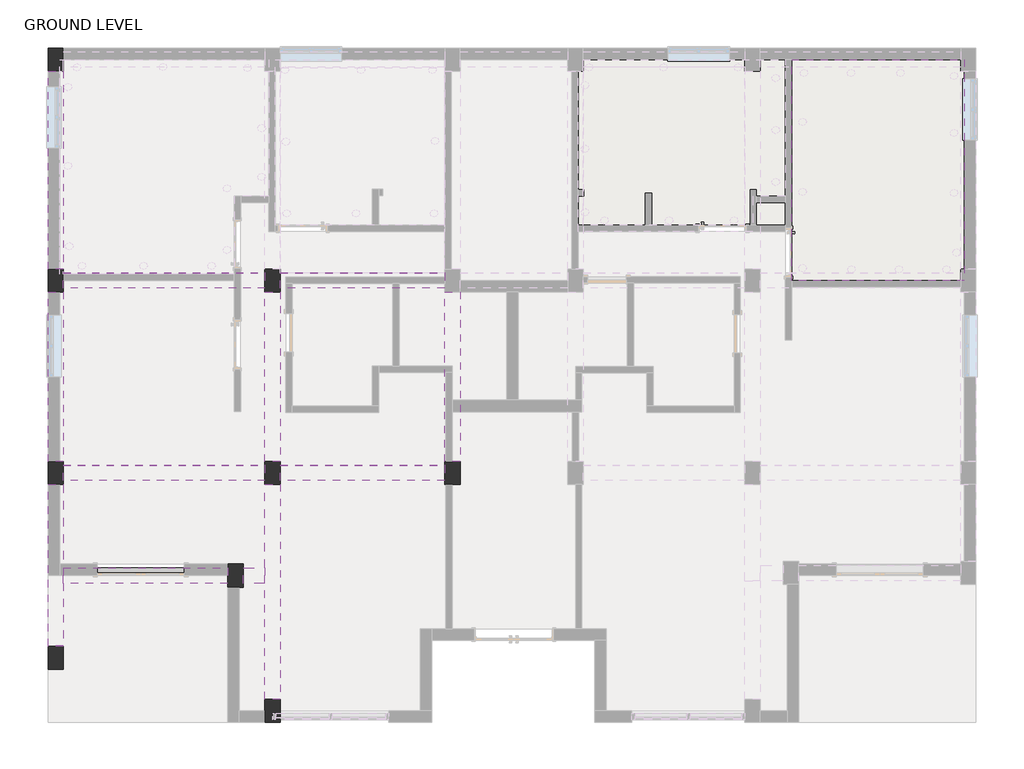
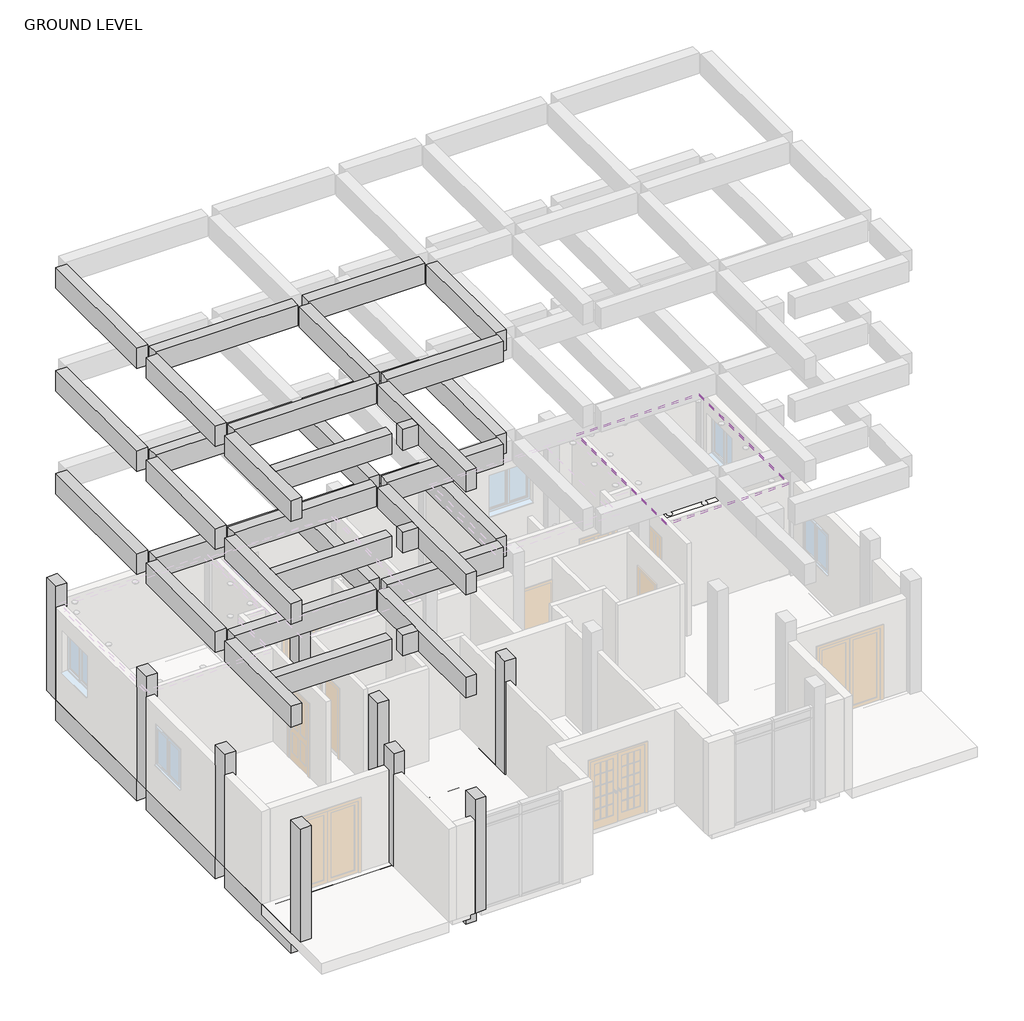
# One storey, part 3 of 5: 48 beams, 9 columns, 2 coverings, 1 slab.
"""IFC4 building model written with IfcOpenShell, lengths in millimetres."""

from ifc_helpers import new_model, si_unit, frame, origin, origin_with_axes, place, context, project, spatial, polyline, outline, extrude, faceted_brep, element, save

model = new_model("IFC4")

# Units and contexts
model_context = context("Model", 3, world=origin())
ifc_project = project(units=[si_unit("LENGTHUNIT", "METRE", prefix="MILLI")], contexts=[model_context])

# Site, building, storey
site = spatial("IfcSite", under=ifc_project)
building = spatial("IfcBuilding", under=site)
storey = spatial("IfcBuildingStorey", under=building, Name="GROUND LEVEL", Elevation=0.0)

# Beams
placement = place(None, origin())
element("IfcBeam", 1, ObjectType="Concrete-Rectangular Beam : 12 x 24", at=placement, inside=storey, context=model_context, shape_type="SweptSolid", body=[
    extrude(outline(polyline([(-8839.9786397, -5600.6620333), (-9144.7786397, -5600.6620333), (-9144.7786397, -1680.8061634), (-8839.9786397, -1680.8061634), (-8839.9786397, -5600.6620333)])), frame((0.0, 0.0, -609.6), z_axis=(0.0, 0.0, 1.0), x_axis=(1.0, 0.0, 0.0)), (0.0, 0.0, 1.0), 609.6),
])
element("IfcBeam", 2, ObjectType="Concrete-Rectangular Beam : 12 x 24", at=placement, inside=storey, context=model_context, shape_type="SweptSolid", body=[
    extrude(outline(polyline([(-8839.9786397, -9410.6620333), (-9144.7786397, -9410.6620333), (-9144.7786397, -6057.8620333), (-8839.9786397, -6057.8620333), (-8839.9786397, -9410.6620333)])), frame((0.0, 0.0, -609.6), z_axis=(0.0, 0.0, 1.0), x_axis=(1.0, 0.0, 0.0)), (0.0, 0.0, 1.0), 609.6),
])
element("IfcBeam", 3, ObjectType="Concrete-Rectangular Beam : 12 x 24", at=placement, inside=storey, context=model_context, shape_type="Brep", body=[
    faceted_brep([(-9144.7786397, -13068.2620333, 0.0), (-8839.9786397, -13068.2620333, 0.0), (-8839.9786397, -11823.6620333, 0.0), (-8839.9786397, -11518.8620333, 0.0), (-8839.9786397, -9867.8620333, 0.0), (-9144.7786397, -9867.8620333, 0.0), (-9144.7786397, -13068.2620333, -609.6), (-9144.7786397, -9867.8620333, -609.6), (-8839.9786397, -13068.2620333, -609.6), (-8839.9786397, -9867.8620333, -609.6), (-8839.9786397, -11518.8620333, -609.6), (-8839.9786397, -11823.6620333, -609.6)], [[[0, 1, 2, 3, 4, 5]], [[6, 0, 5, 7]], [[8, 6, 7, 9, 10, 11]], [[1, 8, 11, 10, 9, 4, 3, 2]], [[4, 9, 7, 5]], [[1, 0, 6, 8]]]),
])
element("IfcBeam", 4, ObjectType="Concrete-Rectangular Beam : 12 x 24", at=placement, inside=storey, context=model_context, shape_type="SweptSolid", body=[
    extrude(outline(polyline([(-4548.1175798, -5981.6620333), (-4548.1175798, -5676.8620333), (-1296.9175798, -5676.8620333), (-1296.9175798, -5981.6620333), (-4548.1175798, -5981.6620333)])), frame((0.0, 0.0, -609.6), z_axis=(0.0, 0.0, 1.0), x_axis=(1.0, 0.0, 0.0)), (0.0, 0.0, 1.0), 609.6),
])
element("IfcBeam", 5, ObjectType="Concrete-Rectangular Beam : 12 x 24", at=placement, inside=storey, context=model_context, shape_type="SweptSolid", body=[
    extrude(outline(polyline([(-8839.9786397, -5981.6620333), (-8839.9786397, -5676.8620333), (-4852.9175798, -5676.8620333), (-4852.9175798, -5981.6620333), (-8839.9786397, -5981.6620333)])), frame((0.0, 0.0, -609.6), z_axis=(0.0, 0.0, 1.0), x_axis=(1.0, 0.0, 0.0)), (0.0, 0.0, 1.0), 609.6),
])
element("IfcBeam", 6, ObjectType="Concrete-Rectangular Beam : 12 x 24", at=placement, inside=storey, context=model_context, shape_type="SweptSolid", body=[
    extrude(outline(polyline([(-4852.9175798, -9486.8620333), (-4852.9175798, -9791.6620333), (-8839.9786397, -9791.6620333), (-8839.9786397, -9486.8620333), (-4852.9175798, -9486.8620333)])), frame((0.0, 0.0, -609.6), z_axis=(0.0, 0.0, 1.0), x_axis=(1.0, 0.0, 0.0)), (0.0, 0.0, 1.0), 609.6),
])
element("IfcBeam", 7, ObjectType="Concrete-Rectangular Beam : 12 x 24", at=placement, inside=storey, context=model_context, shape_type="SweptSolid", body=[
    extrude(outline(polyline([(-1296.9175798, -9486.8620333), (-1296.9175798, -9791.6620333), (-4548.1175798, -9791.6620333), (-4548.1175798, -9486.8620333), (-1296.9175798, -9486.8620333)])), frame((0.0, 0.0, -609.6), z_axis=(0.0, 0.0, 1.0), x_axis=(1.0, 0.0, 0.0)), (0.0, 0.0, 1.0), 609.6),
])
element("IfcBeam", 8, ObjectType="Concrete-Rectangular Beam : 12 x 24", at=placement, inside=storey, context=model_context, shape_type="Brep", body=[
    faceted_brep([(-4852.9175798, -14119.6402089, 0.0), (-4548.1175798, -14119.6402089, 0.0), (-4548.1175798, -9867.8620333, 0.0), (-4852.9175798, -9867.8620333, 0.0), (-4852.9175798, -11518.8620333, 0.0), (-4852.9175798, -11823.6620333, 0.0), (-4852.9175798, -14119.6402089, -609.6), (-4852.9175798, -9867.8620333, -609.6), (-4852.9175798, -11518.8620333, -609.6), (-4852.9175798, -11823.6620333, -609.6), (-4548.1175798, -14119.6402089, -609.6), (-4548.1175798, -9867.8620333, -609.6)], [[[0, 1, 2, 3, 4, 5]], [[6, 0, 5, 4, 3, 7, 8, 9]], [[10, 6, 9, 8, 7, 11]], [[1, 10, 11, 2]], [[2, 11, 7, 3]], [[1, 0, 6, 10]]]),
])
element("IfcBeam", 9, ObjectType="Concrete-Rectangular Beam : 12 x 24", at=placement, inside=storey, context=model_context, shape_type="SweptSolid", body=[
    extrude(outline(polyline([(-5284.7175798, -11823.6620333), (-5284.7175798, -11518.8620333), (-4852.9175798, -11518.8620333), (-4852.9175798, -11823.6620333), (-5284.7175798, -11823.6620333)])), frame((0.0, 0.0, -609.6), z_axis=(0.0, 0.0, 1.0), x_axis=(1.0, 0.0, 0.0)), (0.0, 0.0, 1.0), 609.6),
])
element("IfcBeam", 10, ObjectType="Concrete-Rectangular Beam : 12 x 24", at=placement, inside=storey, context=model_context, shape_type="SweptSolid", body=[
    extrude(outline(polyline([(-5589.5175798, -11518.8620333), (-5589.5175798, -11823.6620333), (-8839.9786397, -11823.6620333), (-8839.9786397, -11518.8620333), (-5589.5175798, -11518.8620333)])), frame((0.0, 0.0, -609.6), z_axis=(0.0, 0.0, 1.0), x_axis=(1.0, 0.0, 0.0)), (0.0, 0.0, 1.0), 609.6),
])
element("IfcBeam", 11, ObjectType="Concrete-Rectangular Beam : 12 x 24", at=placement, inside=storey, context=model_context, shape_type="SweptSolid", body=[
    extrude(outline(polyline([(-4548.1175798, -9410.6620333), (-4852.9175798, -9410.6620333), (-4852.9175798, -6057.8620333), (-4548.1175798, -6057.8620333), (-4548.1175798, -9410.6620333)])), frame((0.0, 0.0, -609.6), z_axis=(0.0, 0.0, 1.0), x_axis=(1.0, 0.0, 0.0)), (0.0, 0.0, 1.0), 609.6),
])
element("IfcBeam", 12, ObjectType="Concrete-Rectangular Beam : 12 x 24", at=placement, inside=storey, context=model_context, shape_type="SweptSolid", body=[
    extrude(outline(polyline([(-992.1175798, -9410.6620333), (-1296.9175798, -9410.6620333), (-1296.9175798, -6057.8620333), (-992.1175798, -6057.8620333), (-992.1175798, -9410.6620333)])), frame((0.0, 0.0, -609.6), z_axis=(0.0, 0.0, 1.0), x_axis=(1.0, 0.0, 0.0)), (0.0, 0.0, 1.0), 609.6),
])
element("IfcBeam", 13, ObjectType="Concrete-Rectangular Beam : 12 x 24", at=placement, inside=storey, context=model_context, shape_type="Brep", body=[
    faceted_brep([(-9144.7786397, -5600.6620333, 6705.6), (-8839.9786397, -5600.6620333, 6705.6), (-8839.9786397, -1680.8061634, 6705.6), (-9144.7786397, -1680.8061634, 6705.6), (-9144.7786397, -5600.6620333, 6096.0), (-9144.7786397, -5600.6620333, 6400.8), (-9144.7786397, -1680.8061634, 6400.8), (-9144.7786397, -1680.8061634, 6096.0), (-8839.9786397, -5600.6620333, 6096.0), (-8839.9786397, -1680.8061634, 6096.0), (-8839.9786397, -5600.6620333, 6400.8), (-8839.9786397, -1680.8061634, 6400.8)], [[[0, 1, 2, 3]], [[4, 5, 0, 3, 6, 7]], [[8, 4, 7, 9]], [[1, 10, 8, 9, 11, 2]], [[2, 11, 9, 7, 6, 3]], [[1, 0, 5, 4, 8, 10]]]),
])
element("IfcBeam", 14, ObjectType="Concrete-Rectangular Beam : 12 x 24", at=placement, inside=storey, context=model_context, shape_type="Brep", body=[
    faceted_brep([(-9144.7786397, -9410.6620333, 6705.6), (-8839.9786397, -9410.6620333, 6705.6), (-8839.9786397, -6057.8620333, 6705.6), (-9144.7786397, -6057.8620333, 6705.6), (-9144.7786397, -9410.6620333, 6096.0), (-9144.7786397, -9410.6620333, 6400.8), (-9144.7786397, -6057.8620333, 6400.8), (-9144.7786397, -6057.8620333, 6096.0), (-8839.9786397, -9410.6620333, 6096.0), (-8839.9786397, -6057.8620333, 6096.0), (-8839.9786397, -9410.6620333, 6400.8), (-8839.9786397, -6057.8620333, 6400.8)], [[[0, 1, 2, 3]], [[4, 5, 0, 3, 6, 7]], [[8, 4, 7, 9]], [[1, 10, 8, 9, 11, 2]], [[2, 11, 9, 7, 6, 3]], [[1, 0, 5, 4, 8, 10]]]),
])
element("IfcBeam", 15, ObjectType="Concrete-Rectangular Beam : 12 x 24", at=placement, inside=storey, context=model_context, shape_type="Brep", body=[
    faceted_brep([(-9144.7786397, -13068.2620333, 6705.6), (-8839.9786397, -13068.2620333, 6705.6), (-8839.9786397, -11823.6620333, 6705.6), (-8839.9786397, -11518.8620333, 6705.6), (-8839.9786397, -9867.8620333, 6705.6), (-9144.7786397, -9867.8620333, 6705.6), (-9144.7786397, -13068.2620333, 6096.0), (-9144.7786397, -13068.2620333, 6400.8), (-9144.7786397, -9867.8620333, 6400.8), (-9144.7786397, -9867.8620333, 6096.0), (-8839.9786397, -13068.2620333, 6096.0), (-8839.9786397, -9867.8620333, 6096.0), (-8839.9786397, -11518.8620333, 6096.0), (-8839.9786397, -11823.6620333, 6096.0), (-8839.9786397, -13068.2620333, 6400.8), (-8839.9786397, -9867.8620333, 6400.8)], [[[0, 1, 2, 3, 4, 5]], [[6, 7, 0, 5, 8, 9]], [[10, 6, 9, 11, 12, 13]], [[1, 14, 10, 13, 12, 11, 15, 4, 3, 2]], [[4, 15, 11, 9, 8, 5]], [[1, 0, 7, 6, 10, 14]]]),
])
element("IfcBeam", 16, ObjectType="Concrete-Rectangular Beam : 12 x 24", at=placement, inside=storey, context=model_context, shape_type="SweptSolid", body=[
    extrude(outline(polyline([(-4548.1175798, -5981.6620333), (-4548.1175798, -5676.8620333), (-1296.9175798, -5676.8620333), (-1296.9175798, -5981.6620333), (-4548.1175798, -5981.6620333)])), frame((0.0, 0.0, 6096.0), z_axis=(0.0, 0.0, 1.0), x_axis=(1.0, 0.0, 0.0)), (0.0, 0.0, 1.0), 609.6),
])
element("IfcBeam", 17, ObjectType="Concrete-Rectangular Beam : 12 x 24", at=placement, inside=storey, context=model_context, shape_type="SweptSolid", body=[
    extrude(outline(polyline([(-8839.9786397, -5981.6620333), (-8839.9786397, -5676.8620333), (-4852.9175798, -5676.8620333), (-4852.9175798, -5981.6620333), (-8839.9786397, -5981.6620333)])), frame((0.0, 0.0, 6096.0), z_axis=(0.0, 0.0, 1.0), x_axis=(1.0, 0.0, 0.0)), (0.0, 0.0, 1.0), 609.6),
])
element("IfcBeam", 18, ObjectType="Concrete-Rectangular Beam : 12 x 24", at=placement, inside=storey, context=model_context, shape_type="SweptSolid", body=[
    extrude(outline(polyline([(-4852.9175798, -9486.8620333), (-4852.9175798, -9791.6620333), (-8839.9786397, -9791.6620333), (-8839.9786397, -9486.8620333), (-4852.9175798, -9486.8620333)])), frame((0.0, 0.0, 6096.0), z_axis=(0.0, 0.0, 1.0), x_axis=(1.0, 0.0, 0.0)), (0.0, 0.0, 1.0), 609.6),
])
element("IfcBeam", 19, ObjectType="Concrete-Rectangular Beam : 12 x 24", at=placement, inside=storey, context=model_context, shape_type="SweptSolid", body=[
    extrude(outline(polyline([(-1296.9175798, -9486.8620333), (-1296.9175798, -9791.6620333), (-4548.1175798, -9791.6620333), (-4548.1175798, -9486.8620333), (-1296.9175798, -9486.8620333)])), frame((0.0, 0.0, 6096.0), z_axis=(0.0, 0.0, 1.0), x_axis=(1.0, 0.0, 0.0)), (0.0, 0.0, 1.0), 609.6),
])
element("IfcBeam", 20, ObjectType="Concrete-Rectangular Beam : 12 x 24", at=placement, inside=storey, context=model_context, shape_type="Brep", body=[
    faceted_brep([(-4852.9175798, -14119.6402089, 6705.6), (-4548.1175798, -14119.6402089, 6705.6), (-4548.1175798, -9867.8620333, 6705.6), (-4852.9175798, -9867.8620333, 6705.6), (-4852.9175798, -11518.8620333, 6705.6), (-4852.9175798, -11823.6620333, 6705.6), (-4852.9175798, -14119.6402089, 6096.0), (-4852.9175798, -14119.6402089, 6400.8), (-4852.9175798, -9867.8620333, 6400.8), (-4852.9175798, -9867.8620333, 6096.0), (-4852.9175798, -11518.8620333, 6096.0), (-4852.9175798, -11823.6620333, 6096.0), (-4548.1175798, -14119.6402089, 6096.0), (-4548.1175798, -9867.8620333, 6096.0), (-4548.1175798, -14119.6402089, 6400.8), (-4548.1175798, -9867.8620333, 6400.8)], [[[0, 1, 2, 3, 4, 5]], [[6, 7, 0, 5, 4, 3, 8, 9, 10, 11]], [[12, 6, 11, 10, 9, 13]], [[1, 14, 12, 13, 15, 2]], [[2, 15, 13, 9, 8, 3]], [[1, 0, 7, 6, 12, 14]]]),
])
element("IfcBeam", 21, ObjectType="Concrete-Rectangular Beam : 12 x 24", at=placement, inside=storey, context=model_context, shape_type="SweptSolid", body=[
    extrude(outline(polyline([(-5284.7175798, -11823.6620333), (-5284.7175798, -11518.8620333), (-4852.9175798, -11518.8620333), (-4852.9175798, -11823.6620333), (-5284.7175798, -11823.6620333)])), frame((0.0, 0.0, 6096.0), z_axis=(0.0, 0.0, 1.0), x_axis=(1.0, 0.0, 0.0)), (0.0, 0.0, 1.0), 609.6),
])
element("IfcBeam", 22, ObjectType="Concrete-Rectangular Beam : 12 x 24", at=placement, inside=storey, context=model_context, shape_type="SweptSolid", body=[
    extrude(outline(polyline([(-5589.5175798, -11518.8620333), (-5589.5175798, -11823.6620333), (-8839.9786397, -11823.6620333), (-8839.9786397, -11518.8620333), (-5589.5175798, -11518.8620333)])), frame((0.0, 0.0, 6096.0), z_axis=(0.0, 0.0, 1.0), x_axis=(1.0, 0.0, 0.0)), (0.0, 0.0, 1.0), 609.6),
])
element("IfcBeam", 23, ObjectType="Concrete-Rectangular Beam : 12 x 24", at=placement, inside=storey, context=model_context, shape_type="Brep", body=[
    faceted_brep([(-4852.9175798, -9410.6620333, 6705.6), (-4548.1175798, -9410.6620333, 6705.6), (-4548.1175798, -6057.8620333, 6705.6), (-4852.9175798, -6057.8620333, 6705.6), (-4852.9175798, -9410.6620333, 6096.0), (-4852.9175798, -9410.6620333, 6400.8), (-4852.9175798, -6057.8620333, 6400.8), (-4852.9175798, -6057.8620333, 6096.0), (-4548.1175798, -9410.6620333, 6096.0), (-4548.1175798, -6057.8620333, 6096.0), (-4548.1175798, -9410.6620333, 6400.8), (-4548.1175798, -6057.8620333, 6400.8)], [[[0, 1, 2, 3]], [[4, 5, 0, 3, 6, 7]], [[8, 4, 7, 9]], [[1, 10, 8, 9, 11, 2]], [[2, 11, 9, 7, 6, 3]], [[1, 0, 5, 4, 8, 10]]]),
])
element("IfcBeam", 24, ObjectType="Concrete-Rectangular Beam : 12 x 24", at=placement, inside=storey, context=model_context, shape_type="Brep", body=[
    faceted_brep([(-1296.9175798, -9410.6620333, 6705.6), (-992.1175798, -9410.6620333, 6705.6), (-992.1175798, -6057.8620333, 6705.6), (-1296.9175798, -6057.8620333, 6705.6), (-1296.9175798, -9410.6620333, 6096.0), (-1296.9175798, -9410.6620333, 6400.8), (-1296.9175798, -6057.8620333, 6400.8), (-1296.9175798, -6057.8620333, 6096.0), (-992.1175798, -9410.6620333, 6096.0), (-992.1175798, -6057.8620333, 6096.0), (-992.1175798, -9410.6620333, 6400.8), (-992.1175798, -6057.8620333, 6400.8)], [[[0, 1, 2, 3]], [[4, 5, 0, 3, 6, 7]], [[8, 4, 7, 9]], [[1, 10, 8, 9, 11, 2]], [[2, 11, 9, 7, 6, 3]], [[1, 0, 5, 4, 8, 10]]]),
])
element("IfcBeam", 25, ObjectType="Concrete-Rectangular Beam : 12 x 24", at=placement, inside=storey, context=model_context, shape_type="Brep", body=[
    faceted_brep([(-9144.7786397, -5600.6620333, 9753.6), (-8839.9786397, -5600.6620333, 9753.6), (-8839.9786397, -1680.8061634, 9753.6), (-9144.7786397, -1680.8061634, 9753.6), (-9144.7786397, -5600.6620333, 9144.0), (-9144.7786397, -5600.6620333, 9448.8), (-9144.7786397, -1680.8061634, 9448.8), (-9144.7786397, -1680.8061634, 9144.0), (-8839.9786397, -5600.6620333, 9144.0), (-8839.9786397, -1680.8061634, 9144.0), (-8839.9786397, -5600.6620333, 9448.8), (-8839.9786397, -1680.8061634, 9448.8)], [[[0, 1, 2, 3]], [[4, 5, 0, 3, 6, 7]], [[8, 4, 7, 9]], [[1, 10, 8, 9, 11, 2]], [[2, 11, 9, 7, 6, 3]], [[1, 0, 5, 4, 8, 10]]]),
])
element("IfcBeam", 26, ObjectType="Concrete-Rectangular Beam : 12 x 24", at=placement, inside=storey, context=model_context, shape_type="Brep", body=[
    faceted_brep([(-9144.7786397, -9410.6620333, 9753.6), (-8839.9786397, -9410.6620333, 9753.6), (-8839.9786397, -6057.8620333, 9753.6), (-9144.7786397, -6057.8620333, 9753.6), (-9144.7786397, -9410.6620333, 9144.0), (-9144.7786397, -9410.6620333, 9448.8), (-9144.7786397, -6057.8620333, 9448.8), (-9144.7786397, -6057.8620333, 9144.0), (-8839.9786397, -9410.6620333, 9144.0), (-8839.9786397, -6057.8620333, 9144.0), (-8839.9786397, -9410.6620333, 9448.8), (-8839.9786397, -6057.8620333, 9448.8)], [[[0, 1, 2, 3]], [[4, 5, 0, 3, 6, 7]], [[8, 4, 7, 9]], [[1, 10, 8, 9, 11, 2]], [[2, 11, 9, 7, 6, 3]], [[1, 0, 5, 4, 8, 10]]]),
])
element("IfcBeam", 27, ObjectType="Concrete-Rectangular Beam : 12 x 24", at=placement, inside=storey, context=model_context, shape_type="Brep", body=[
    faceted_brep([(-9144.7786397, -13068.2620333, 9753.6), (-8839.9786397, -13068.2620333, 9753.6), (-8839.9786397, -11823.6620333, 9753.6), (-8839.9786397, -11518.8620333, 9753.6), (-8839.9786397, -9867.8620333, 9753.6), (-9144.7786397, -9867.8620333, 9753.6), (-9144.7786397, -13068.2620333, 9144.0), (-9144.7786397, -13068.2620333, 9448.8), (-9144.7786397, -9867.8620333, 9448.8), (-9144.7786397, -9867.8620333, 9144.0), (-8839.9786397, -13068.2620333, 9144.0), (-8839.9786397, -9867.8620333, 9144.0), (-8839.9786397, -11518.8620333, 9144.0), (-8839.9786397, -11823.6620333, 9144.0), (-8839.9786397, -13068.2620333, 9448.8), (-8839.9786397, -9867.8620333, 9448.8)], [[[0, 1, 2, 3, 4, 5]], [[6, 7, 0, 5, 8, 9]], [[10, 6, 9, 11, 12, 13]], [[1, 14, 10, 13, 12, 11, 15, 4, 3, 2]], [[4, 15, 11, 9, 8, 5]], [[1, 0, 7, 6, 10, 14]]]),
])
element("IfcBeam", 28, ObjectType="Concrete-Rectangular Beam : 12 x 24", at=placement, inside=storey, context=model_context, shape_type="SweptSolid", body=[
    extrude(outline(polyline([(-4548.1175798, -5981.6620333), (-4548.1175798, -5676.8620333), (-1296.9175798, -5676.8620333), (-1296.9175798, -5981.6620333), (-4548.1175798, -5981.6620333)])), frame((0.0, 0.0, 9144.0), z_axis=(0.0, 0.0, 1.0), x_axis=(1.0, 0.0, 0.0)), (0.0, 0.0, 1.0), 609.6),
])
element("IfcBeam", 29, ObjectType="Concrete-Rectangular Beam : 12 x 24", at=placement, inside=storey, context=model_context, shape_type="SweptSolid", body=[
    extrude(outline(polyline([(-8839.9786397, -5981.6620333), (-8839.9786397, -5676.8620333), (-4852.9175798, -5676.8620333), (-4852.9175798, -5981.6620333), (-8839.9786397, -5981.6620333)])), frame((0.0, 0.0, 9144.0), z_axis=(0.0, 0.0, 1.0), x_axis=(1.0, 0.0, 0.0)), (0.0, 0.0, 1.0), 609.6),
])
element("IfcBeam", 30, ObjectType="Concrete-Rectangular Beam : 12 x 24", at=placement, inside=storey, context=model_context, shape_type="SweptSolid", body=[
    extrude(outline(polyline([(-4852.9175798, -9486.8620333), (-4852.9175798, -9791.6620333), (-8839.9786397, -9791.6620333), (-8839.9786397, -9486.8620333), (-4852.9175798, -9486.8620333)])), frame((0.0, 0.0, 9144.0), z_axis=(0.0, 0.0, 1.0), x_axis=(1.0, 0.0, 0.0)), (0.0, 0.0, 1.0), 609.6),
])
element("IfcBeam", 31, ObjectType="Concrete-Rectangular Beam : 12 x 24", at=placement, inside=storey, context=model_context, shape_type="SweptSolid", body=[
    extrude(outline(polyline([(-1296.9175798, -9486.8620333), (-1296.9175798, -9791.6620333), (-4548.1175798, -9791.6620333), (-4548.1175798, -9486.8620333), (-1296.9175798, -9486.8620333)])), frame((0.0, 0.0, 9144.0), z_axis=(0.0, 0.0, 1.0), x_axis=(1.0, 0.0, 0.0)), (0.0, 0.0, 1.0), 609.6),
])
element("IfcBeam", 32, ObjectType="Concrete-Rectangular Beam : 12 x 24", at=placement, inside=storey, context=model_context, shape_type="Brep", body=[
    faceted_brep([(-4852.9175798, -14119.6402089, 9753.6), (-4548.1175798, -14119.6402089, 9753.6), (-4548.1175798, -9867.8620333, 9753.6), (-4852.9175798, -9867.8620333, 9753.6), (-4852.9175798, -11518.8620333, 9753.6), (-4852.9175798, -11823.6620333, 9753.6), (-4852.9175798, -14119.6402089, 9144.0), (-4852.9175798, -14119.6402089, 9448.8), (-4852.9175798, -9867.8620333, 9448.8), (-4852.9175798, -9867.8620333, 9144.0), (-4852.9175798, -11518.8620333, 9144.0), (-4852.9175798, -11823.6620333, 9144.0), (-4548.1175798, -14119.6402089, 9144.0), (-4548.1175798, -9867.8620333, 9144.0), (-4548.1175798, -14119.6402089, 9448.8), (-4548.1175798, -9867.8620333, 9448.8)], [[[0, 1, 2, 3, 4, 5]], [[6, 7, 0, 5, 4, 3, 8, 9, 10, 11]], [[12, 6, 11, 10, 9, 13]], [[1, 14, 12, 13, 15, 2]], [[2, 15, 13, 9, 8, 3]], [[1, 0, 7, 6, 12, 14]]]),
])
element("IfcBeam", 33, ObjectType="Concrete-Rectangular Beam : 12 x 24", at=placement, inside=storey, context=model_context, shape_type="SweptSolid", body=[
    extrude(outline(polyline([(-5284.7175798, -11823.6620333), (-5284.7175798, -11518.8620333), (-4852.9175798, -11518.8620333), (-4852.9175798, -11823.6620333), (-5284.7175798, -11823.6620333)])), frame((0.0, 0.0, 9144.0), z_axis=(0.0, 0.0, 1.0), x_axis=(1.0, 0.0, 0.0)), (0.0, 0.0, 1.0), 609.6),
])
element("IfcBeam", 34, ObjectType="Concrete-Rectangular Beam : 12 x 24", at=placement, inside=storey, context=model_context, shape_type="SweptSolid", body=[
    extrude(outline(polyline([(-5589.5175798, -11518.8620333), (-5589.5175798, -11823.6620333), (-8839.9786397, -11823.6620333), (-8839.9786397, -11518.8620333), (-5589.5175798, -11518.8620333)])), frame((0.0, 0.0, 9144.0), z_axis=(0.0, 0.0, 1.0), x_axis=(1.0, 0.0, 0.0)), (0.0, 0.0, 1.0), 609.6),
])
element("IfcBeam", 35, ObjectType="Concrete-Rectangular Beam : 12 x 24", at=placement, inside=storey, context=model_context, shape_type="Brep", body=[
    faceted_brep([(-4852.9175798, -9410.6620333, 9753.6), (-4548.1175798, -9410.6620333, 9753.6), (-4548.1175798, -6057.8620333, 9753.6), (-4852.9175798, -6057.8620333, 9753.6), (-4852.9175798, -9410.6620333, 9144.0), (-4852.9175798, -9410.6620333, 9448.8), (-4852.9175798, -6057.8620333, 9448.8), (-4852.9175798, -6057.8620333, 9144.0), (-4548.1175798, -9410.6620333, 9144.0), (-4548.1175798, -6057.8620333, 9144.0), (-4548.1175798, -9410.6620333, 9448.8), (-4548.1175798, -6057.8620333, 9448.8)], [[[0, 1, 2, 3]], [[4, 5, 0, 3, 6, 7]], [[8, 4, 7, 9]], [[1, 10, 8, 9, 11, 2]], [[2, 11, 9, 7, 6, 3]], [[1, 0, 5, 4, 8, 10]]]),
])
element("IfcBeam", 36, ObjectType="Concrete-Rectangular Beam : 12 x 24", at=placement, inside=storey, context=model_context, shape_type="Brep", body=[
    faceted_brep([(-1296.9175798, -9410.6620333, 9753.6), (-992.1175798, -9410.6620333, 9753.6), (-992.1175798, -6057.8620333, 9753.6), (-1296.9175798, -6057.8620333, 9753.6), (-1296.9175798, -9410.6620333, 9144.0), (-1296.9175798, -9410.6620333, 9448.8), (-1296.9175798, -6057.8620333, 9448.8), (-1296.9175798, -6057.8620333, 9144.0), (-992.1175798, -9410.6620333, 9144.0), (-992.1175798, -6057.8620333, 9144.0), (-992.1175798, -9410.6620333, 9448.8), (-992.1175798, -6057.8620333, 9448.8)], [[[0, 1, 2, 3]], [[4, 5, 0, 3, 6, 7]], [[8, 4, 7, 9]], [[1, 10, 8, 9, 11, 2]], [[2, 11, 9, 7, 6, 3]], [[1, 0, 5, 4, 8, 10]]]),
])
element("IfcBeam", 37, ObjectType="Concrete-Rectangular Beam : 12 x 24", at=placement, inside=storey, context=model_context, shape_type="SweptSolid", body=[
    extrude(outline(polyline([(-8839.9786397, -5600.6620333), (-9144.7786397, -5600.6620333), (-9144.7786397, -1680.8061634), (-8839.9786397, -1680.8061634), (-8839.9786397, -5600.6620333)])), frame((0.0, 0.0, 12192.0), z_axis=(0.0, 0.0, 1.0), x_axis=(1.0, 0.0, 0.0)), (0.0, 0.0, 1.0), 609.6),
])
element("IfcBeam", 38, ObjectType="Concrete-Rectangular Beam : 12 x 24", at=placement, inside=storey, context=model_context, shape_type="SweptSolid", body=[
    extrude(outline(polyline([(-8839.9786397, -9410.6620333), (-9144.7786397, -9410.6620333), (-9144.7786397, -6057.8620333), (-8839.9786397, -6057.8620333), (-8839.9786397, -9410.6620333)])), frame((0.0, 0.0, 12192.0), z_axis=(0.0, 0.0, 1.0), x_axis=(1.0, 0.0, 0.0)), (0.0, 0.0, 1.0), 609.6),
])
element("IfcBeam", 39, ObjectType="Concrete-Rectangular Beam : 12 x 24", at=placement, inside=storey, context=model_context, shape_type="Brep", body=[
    faceted_brep([(-9144.7786397, -13068.2620333, 12801.6), (-8839.9786397, -13068.2620333, 12801.6), (-8839.9786397, -11823.6620333, 12801.6), (-8839.9786397, -11518.8620333, 12801.6), (-8839.9786397, -9867.8620333, 12801.6), (-9144.7786397, -9867.8620333, 12801.6), (-9144.7786397, -13068.2620333, 12192.0), (-9144.7786397, -9867.8620333, 12192.0), (-8839.9786397, -13068.2620333, 12192.0), (-8839.9786397, -9867.8620333, 12192.0), (-8839.9786397, -11518.8620333, 12192.0), (-8839.9786397, -11823.6620333, 12192.0)], [[[0, 1, 2, 3, 4, 5]], [[6, 0, 5, 7]], [[8, 6, 7, 9, 10, 11]], [[1, 8, 11, 10, 9, 4, 3, 2]], [[4, 9, 7, 5]], [[1, 0, 6, 8]]]),
])
element("IfcBeam", 40, ObjectType="Concrete-Rectangular Beam : 12 x 24", at=placement, inside=storey, context=model_context, shape_type="SweptSolid", body=[
    extrude(outline(polyline([(-4548.1175798, -5981.6620333), (-4548.1175798, -5676.8620333), (-1296.9175798, -5676.8620333), (-1296.9175798, -5981.6620333), (-4548.1175798, -5981.6620333)])), frame((0.0, 0.0, 12192.0), z_axis=(0.0, 0.0, 1.0), x_axis=(1.0, 0.0, 0.0)), (0.0, 0.0, 1.0), 609.6),
])
element("IfcBeam", 41, ObjectType="Concrete-Rectangular Beam : 12 x 24", at=placement, inside=storey, context=model_context, shape_type="SweptSolid", body=[
    extrude(outline(polyline([(-8839.9786397, -5981.6620333), (-8839.9786397, -5676.8620333), (-4852.9175798, -5676.8620333), (-4852.9175798, -5981.6620333), (-8839.9786397, -5981.6620333)])), frame((0.0, 0.0, 12192.0), z_axis=(0.0, 0.0, 1.0), x_axis=(1.0, 0.0, 0.0)), (0.0, 0.0, 1.0), 609.6),
])
element("IfcBeam", 42, ObjectType="Concrete-Rectangular Beam : 12 x 24", at=placement, inside=storey, context=model_context, shape_type="SweptSolid", body=[
    extrude(outline(polyline([(-4852.9175798, -9486.8620333), (-4852.9175798, -9791.6620333), (-8839.9786397, -9791.6620333), (-8839.9786397, -9486.8620333), (-4852.9175798, -9486.8620333)])), frame((0.0, 0.0, 12192.0), z_axis=(0.0, 0.0, 1.0), x_axis=(1.0, 0.0, 0.0)), (0.0, 0.0, 1.0), 609.6),
])
element("IfcBeam", 43, ObjectType="Concrete-Rectangular Beam : 12 x 24", at=placement, inside=storey, context=model_context, shape_type="SweptSolid", body=[
    extrude(outline(polyline([(-1296.9175798, -9486.8620333), (-1296.9175798, -9791.6620333), (-4548.1175798, -9791.6620333), (-4548.1175798, -9486.8620333), (-1296.9175798, -9486.8620333)])), frame((0.0, 0.0, 12192.0), z_axis=(0.0, 0.0, 1.0), x_axis=(1.0, 0.0, 0.0)), (0.0, 0.0, 1.0), 609.6),
])
element("IfcBeam", 44, ObjectType="Concrete-Rectangular Beam : 12 x 24", at=placement, inside=storey, context=model_context, shape_type="Brep", body=[
    faceted_brep([(-4852.9175798, -14119.6402089, 12801.6), (-4548.1175798, -14119.6402089, 12801.6), (-4548.1175798, -9867.8620333, 12801.6), (-4852.9175798, -9867.8620333, 12801.6), (-4852.9175798, -11518.8620333, 12801.6), (-4852.9175798, -11823.6620333, 12801.6), (-4852.9175798, -14119.6402089, 12192.0), (-4852.9175798, -9867.8620333, 12192.0), (-4852.9175798, -11518.8620333, 12192.0), (-4852.9175798, -11823.6620333, 12192.0), (-4548.1175798, -14119.6402089, 12192.0), (-4548.1175798, -9867.8620333, 12192.0)], [[[0, 1, 2, 3, 4, 5]], [[6, 0, 5, 4, 3, 7, 8, 9]], [[10, 6, 9, 8, 7, 11]], [[1, 10, 11, 2]], [[2, 11, 7, 3]], [[1, 0, 6, 10]]]),
])
element("IfcBeam", 45, ObjectType="Concrete-Rectangular Beam : 12 x 24", at=placement, inside=storey, context=model_context, shape_type="SweptSolid", body=[
    extrude(outline(polyline([(-5284.7175798, -11823.6620333), (-5284.7175798, -11518.8620333), (-4852.9175798, -11518.8620333), (-4852.9175798, -11823.6620333), (-5284.7175798, -11823.6620333)])), frame((0.0, 0.0, 12192.0), z_axis=(0.0, 0.0, 1.0), x_axis=(1.0, 0.0, 0.0)), (0.0, 0.0, 1.0), 609.6),
])
element("IfcBeam", 46, ObjectType="Concrete-Rectangular Beam : 12 x 24", at=placement, inside=storey, context=model_context, shape_type="SweptSolid", body=[
    extrude(outline(polyline([(-5589.5175798, -11518.8620333), (-5589.5175798, -11823.6620333), (-8839.9786397, -11823.6620333), (-8839.9786397, -11518.8620333), (-5589.5175798, -11518.8620333)])), frame((0.0, 0.0, 12192.0), z_axis=(0.0, 0.0, 1.0), x_axis=(1.0, 0.0, 0.0)), (0.0, 0.0, 1.0), 609.6),
])
element("IfcBeam", 47, ObjectType="Concrete-Rectangular Beam : 12 x 24", at=placement, inside=storey, context=model_context, shape_type="SweptSolid", body=[
    extrude(outline(polyline([(-4548.1175798, -9410.6620333), (-4852.9175798, -9410.6620333), (-4852.9175798, -6057.8620333), (-4548.1175798, -6057.8620333), (-4548.1175798, -9410.6620333)])), frame((0.0, 0.0, 12192.0), z_axis=(0.0, 0.0, 1.0), x_axis=(1.0, 0.0, 0.0)), (0.0, 0.0, 1.0), 609.6),
])
element("IfcBeam", 48, ObjectType="Concrete-Rectangular Beam : 12 x 24", at=placement, inside=storey, context=model_context, shape_type="SweptSolid", body=[
    extrude(outline(polyline([(-992.1175798, -9410.6620333), (-1296.9175798, -9410.6620333), (-1296.9175798, -6057.8620333), (-992.1175798, -6057.8620333), (-992.1175798, -9410.6620333)])), frame((0.0, 0.0, 12192.0), z_axis=(0.0, 0.0, 1.0), x_axis=(1.0, 0.0, 0.0)), (0.0, 0.0, 1.0), 609.6),
])

# Columns
element("IfcColumn", 49, ObjectType="Concrete-Rectangular-Column : 1'6\" X 1' COLUMN", at=placement, inside=storey, context=model_context, shape_type="SweptSolid", body=[
    extrude(outline(polyline([(-8839.9786397, -1223.6061634), (-8839.9786397, -1680.8061634), (-9144.7786397, -1680.8061634), (-9144.7786397, -1223.6061634), (-8839.9786397, -1223.6061634)])), origin_with_axes(), (0.0, 0.0, 1.0), 3352.8),
])
element("IfcColumn", 50, ObjectType="Concrete-Rectangular-Column : 1'6\" X 1' COLUMN", at=placement, inside=storey, context=model_context, shape_type="SweptSolid", body=[
    extrude(outline(polyline([(-4548.1175798, -5600.6620333), (-4548.1175798, -6057.8620333), (-4852.9175798, -6057.8620333), (-4852.9175798, -5600.6620333), (-4548.1175798, -5600.6620333)])), origin_with_axes(), (0.0, 0.0, 1.0), 3352.8),
])
element("IfcColumn", 51, ObjectType="Concrete-Rectangular-Column : 1'6\" X 1' COLUMN", at=placement, inside=storey, context=model_context, shape_type="SweptSolid", body=[
    extrude(outline(polyline([(-8839.9786397, -5600.6620333), (-8839.9786397, -6057.8620333), (-9144.7786397, -6057.8620333), (-9144.7786397, -5600.6620333), (-8839.9786397, -5600.6620333)])), origin_with_axes(), (0.0, 0.0, 1.0), 3352.8),
])
element("IfcColumn", 52, ObjectType="Concrete-Rectangular-Column : 1'6\" X 1' COLUMN", at=placement, inside=storey, context=model_context, shape_type="SweptSolid", body=[
    extrude(outline(polyline([(-8839.9786397, -9410.6620333), (-8839.9786397, -9867.8620333), (-9144.7786397, -9867.8620333), (-9144.7786397, -9410.6620333), (-8839.9786397, -9410.6620333)])), origin_with_axes(), (0.0, 0.0, 1.0), 3352.8),
])
element("IfcColumn", 53, ObjectType="Concrete-Rectangular-Column : 1'6\" X 1' COLUMN", at=placement, inside=storey, context=model_context, shape_type="SweptSolid", body=[
    extrude(outline(polyline([(-4548.1175798, -9410.6620333), (-4548.1175798, -9867.8620333), (-4852.9175798, -9867.8620333), (-4852.9175798, -9410.6620333), (-4548.1175798, -9410.6620333)])), origin_with_axes(), (0.0, 0.0, 1.0), 3352.8),
])
element("IfcColumn", 54, ObjectType="Concrete-Rectangular-Column : 1'6\" X 1' COLUMN", at=placement, inside=storey, context=model_context, shape_type="SweptSolid", body=[
    extrude(outline(polyline([(-992.1175798, -9410.6620333), (-992.1175798, -9867.8620333), (-1296.9175798, -9867.8620333), (-1296.9175798, -9410.6620333), (-992.1175798, -9410.6620333)])), origin_with_axes(), (0.0, 0.0, 1.0), 3352.8),
])
element("IfcColumn", 55, ObjectType="Concrete-Rectangular-Column : 1'6\" X 1' COLUMN", at=placement, inside=storey, context=model_context, shape_type="SweptSolid", body=[
    extrude(outline(polyline([(-4548.1175798, -14119.6402089), (-4548.1175798, -14576.8402089), (-4852.9175798, -14576.8402089), (-4852.9175798, -14119.6402089), (-4548.1175798, -14119.6402089)])), origin_with_axes(), (0.0, 0.0, 1.0), 3352.8),
])
element("IfcColumn", 56, ObjectType="Concrete-Rectangular-Column : 1'6\" X 1' COLUMN", at=placement, inside=storey, context=model_context, shape_type="SweptSolid", body=[
    extrude(outline(polyline([(-8839.9786397, -13068.2620333), (-8839.9786397, -13525.4620333), (-9144.7786397, -13525.4620333), (-9144.7786397, -13068.2620333), (-8839.9786397, -13068.2620333)])), origin_with_axes(), (0.0, 0.0, 1.0), 3352.8),
])
element("IfcColumn", 57, ObjectType="Concrete-Rectangular-Column : 1'6\" X 1' COLUMN", at=placement, inside=storey, context=model_context, shape_type="SweptSolid", body=[
    extrude(outline(polyline([(-5284.7175798, -11442.6620333), (-5284.7175798, -11899.8620333), (-5589.5175798, -11899.8620333), (-5589.5175798, -11442.6620333), (-5284.7175798, -11442.6620333)])), origin_with_axes(), (0.0, 0.0, 1.0), 3352.8),
])

# Coverings
element("IfcCovering", 58, ObjectType="white ceiling 6\"", at=placement, inside=storey, context=model_context, shape_type="SweptSolid", body=[
    extrude(outline(polyline([(5573.7824202, -5829.2620333), (5573.7824202, -1452.2061634), (8990.0824202, -1452.2061634), (8990.0824202, -5829.2620333), (5573.7824202, -5829.2620333)])), frame((0.0, 0.0, 2590.8), z_axis=(0.0, 0.0, 1.0), x_axis=(1.0, 0.0, 0.0)), (0.0, 0.0, 1.0), 41.275),
])
element("IfcCovering", 59, ObjectType="white ceiling 6\"", at=placement, inside=storey, context=model_context, shape_type="SweptSolid", body=[
    extrude(outline(polyline([(8990.0824202, -1452.2061634), (8990.0824202, -5829.2620333), (5573.7824202, -5829.2620333), (5573.7824202, -1452.2061634), (8990.0824202, -1452.2061634)]), holes=[polyline([(8609.0824202, -1833.2061634), (5954.7824202, -1833.2061634), (5954.7824202, -5448.2620333), (8609.0824202, -5448.2620333), (8609.0824202, -1833.2061634)])]), frame((0.0, 0.0, 2540.0), z_axis=(0.0, 0.0, 1.0), x_axis=(1.0, 0.0, 0.0)), (0.0, 0.0, 1.0), 41.275),
])

# Slab
element("IfcSlab", 60, ObjectType="flooring 1'", at=placement, inside=storey, context=model_context, shape_type="SweptSolid", body=[
    extrude(outline(polyline([(4646.6824202, -1452.2061634), (4646.6824202, -1680.8061634), (4951.4824202, -1680.8061634), (4951.4824202, -1452.2061634), (5446.7824202, -1452.2061634), (5446.7824202, -4157.3061634), (4875.2824202, -4157.3061634), (4875.2824202, -4030.3061634), (4748.2824202, -4030.3061634), (4748.2824202, -4728.8061634), (2805.1824202, -4728.8061634), (2805.1824202, -4093.8061634), (2678.1824202, -4093.8061634), (2678.1824202, -4728.8061634), (1344.6824202, -4728.8061634), (1344.6824202, -4157.3061634), (1458.9824202, -4157.3061634), (1458.9824202, -4030.3061634), (1344.6824202, -4030.3061634), (1344.6824202, -1680.8061634), (1446.2824202, -1680.8061634), (1446.2824202, -1452.2061634), (4646.6824202, -1452.2061634)])), frame((0.0, 0.0, -304.8), z_axis=(0.0, 0.0, 1.0), x_axis=(1.0, 0.0, 0.0)), (0.0, 0.0, 1.0), 304.8),
    extrude(outline(polyline([(5446.7824202, -4284.3061634), (5446.7824202, -4728.8061634), (4875.2824202, -4728.8061634), (4875.2824202, -4284.3061634), (5446.7824202, -4284.3061634)])), frame((0.0, 0.0, -304.8), z_axis=(0.0, 0.0, 1.0), x_axis=(1.0, 0.0, 0.0)), (0.0, 0.0, 1.0), 304.8),
    extrude(outline(polyline([(8913.8824202, -5829.2620333), (5573.7824202, -5829.2620333), (5573.7824202, -1452.2061634), (8913.8824202, -1452.2061634), (8913.8824202, -1680.8061634), (8990.0824202, -1680.8061634), (8990.0824202, -5600.6620333), (8913.8824202, -5600.6620333), (8913.8824202, -5829.2620333)])), frame((0.0, 0.0, -304.8), z_axis=(0.0, 0.0, 1.0), x_axis=(1.0, 0.0, 0.0)), (0.0, 0.0, 1.0), 304.8),
])

save(model, "model.ifc")

# Revit data of these elements
# Type "Concrete-Rectangular Beam : 12 x 24"
#   Assembly Code = "B10"
#   Length [instance default] = 5' - 0"
#   b = 1' - 0"
#   h = 2' - 0"
#   Structural Material [instance default] = Concrete, Cast-in-Place gray
# Type "Concrete-Rectangular-Column : 1'6\" X 1' COLUMN"
#   Assembly Code = "B10"
#   b = 1' - 0"
#   h = 1' - 6"
#   Structural Material [instance default] = Concrete, Cast-in-Place gray
# Type "white ceiling 6\""
#   Assembly Code = "C3030220"
#   built-in parameter 1002203 = 1 (stored number, unit not read)
#   built-in parameter 1002202 = 1 (stored number, unit not read)
#   Layers, outside or top first: 0' - 1" "white ceiling" (function 1); 0' - 0 5/8" "white ceiling" (function 5)
# Type "flooring 1'"
#   Assembly Code = "B1010"
#   Function = 0
#   Layers, outside or top first: 1' - 0" "FL_MARBLE WHITE" (function 1)
# Elements 1, 2, 3, 4, 5, 6, 7, 8, 9, 10, 11, 12, 13, 14, 15, 16, 17, 18, 19, 20, 21, 22, 23, 24, 25, 26, 27, 28, 29, 30, 31, 32, 33, 34, 35, 36, 37, 38, 39, 40, 41, 42, 43, 44, 45, 46, 47, 48 (IfcBeam, "Concrete-Rectangular Beam : 12 x 24")
#   Structural Material = WARM BEIGE COLOUR
#   Phase Created = New Construction
#   Materials on its faces: "WARM BEIGE COLOUR"
# Elements 49, 50, 51, 52, 53, 54, 55, 56, 57 (IfcColumn, "Concrete-Rectangular-Column : 1'6\" X 1' COLUMN")
#   Structural Material = WARM BEIGE COLOUR
#   Phase Created = New Construction
#   Materials on its faces: "WARM BEIGE COLOUR"
# Element 58 (IfcCovering, "white ceiling 6\"")
#   Height Offset From Level = 8' - 6"
#   Phase Created = New Construction
#   Materials on its faces: "white ceiling"
# Element 59 (IfcCovering, "white ceiling 6\"")
#   Height Offset From Level = 8' - 4"
#   Phase Created = New Construction
#   Materials on its faces: "white ceiling"
# Element 60 (IfcSlab, "flooring 1'")
#   Height Offset From Level = 0' - 0"
#   Phase Created = New Construction
#   Materials on its faces: "FL_MARBLE WHITE"
# Materials
#   "Concrete, Cast-in-Place gray": class "Concrete", colour RGB 192 192 192, transparency 0, Description = "Cast-in-place concrete", Cost = 0
#   "white ceiling": class "Generic", colour RGB 120 120 120, transparency 0, Cost = 0
#   "FL_MARBLE WHITE": class "Generic", colour RGB 120 120 120, transparency 0, Cost = 0
#   "WARM BEIGE COLOUR": class "Generic", colour RGB 120 120 120, transparency 0, Cost = 0
